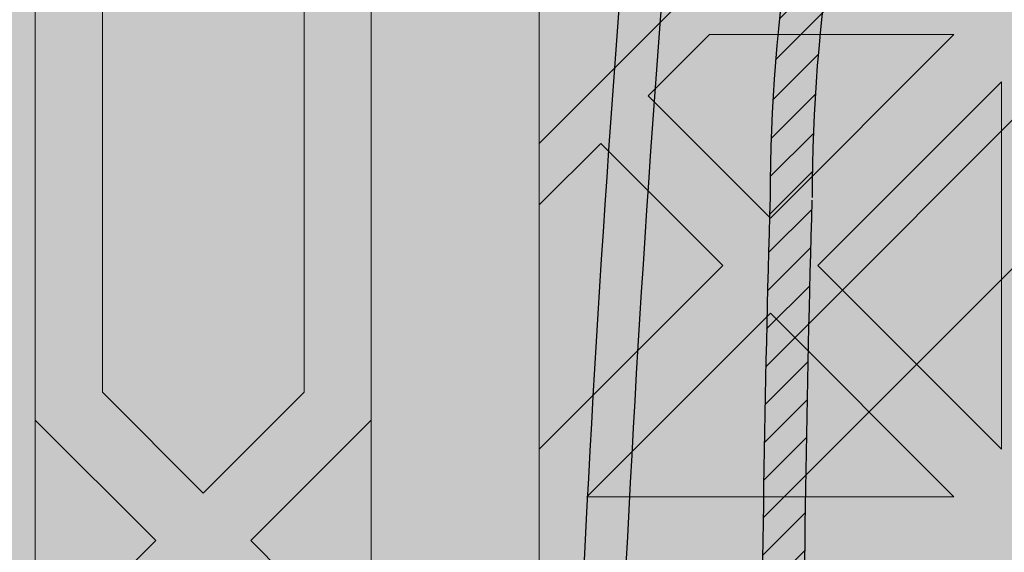
# Model space of a CAD drawing. Units: inches. Extents: x 844 to 2234, y 346 to 1084.
# Tile 16 of 93: x 1116.421 to 1120.159, y 699.229 to 701.25. Entities that reach past the tile are written whole.
import ezdxf

# ---------------------------------------------------------------- set-up
doc = ezdxf.new("R2010")
doc.units = ezdxf.units.IN
doc.header["$MEASUREMENT"] = 0
for name, color, linetype, lineweight in [('A-ANNO-DIMS', 2, 'Continuous', 18), ('furniture', 8, 'Continuous', 18), ('RA-AP-01$0$INT', 35, 'Continuous', 5)]:
    doc.layers.add(name, color=color, linetype=linetype, lineweight=lineweight)
doc.layers.add('RA-AP-01$0$FURN', color=3, linetype='Continuous')
doc.layers.add('RA-AP-01$0$WOOD', color=64, linetype='Continuous')
doc.styles.get("Standard").update_dxf_attribs({"font": 'arial.ttf'})
doc.dimstyles.get("Standard").update_dxf_attribs({"dimtxt": 6, "dimasz": 3, "dimexe": 0.18, "dimexo": 0.0625, "dimgap": 0.09, "dimtad": 0, "dimtih": 1, "dimtoh": 1, "dimdec": 1, "dimzin": 0, "dimdsep": 46, "dimlunit": 3, "dimtxsty": 'Standard', "dimblk": 'ARCHTICK', "dimcen": 0.09, "dimadec": 0, "dimazin": 0, "dimtfac": 1, "dimtdec": 1, "dimtofl": 0, "dimtmove": 0, "dimatfit": 3, "dimfxl": 1, "dimtolj": 1, "dimtzin": 0, "dimarcsym": 0})

# ---------------------------------------------------------------- blocks, each defined once
blk = doc.blocks.new('A$C18D01794')
at = {"layer": 'RA-AP-01$0$INT'}
h = blk.add_hatch(color=256, dxfattribs=at)
h.paths.add_polyline_path([(4.35521, -6.15671), (4.35521, -8.05671), (5.45521, -8.05671), (5.45521, -6.15671)])
h.paths.add_polyline_path([(4.40521, -8.00671), (4.40521, -6.20671), (5.40521, -6.20671), (5.40521, -8.00671)], flags=16)
h = blk.add_hatch(color=256, dxfattribs=at)
h.paths.add_polyline_path([(4.50521, -7.5855), (4.46935, -7.54964), (4.50521, -7.51378), (4.50521, -7.38196), (4.46935, -7.34611), (4.50521, -7.31025), (4.50521, -7.17843), (4.46935, -7.14257), (4.50521, -7.10671), (4.47692, -7.10671), (4.45521, -7.12843), (4.43349, -7.10671), (4.40521, -7.10671), (4.44106, -7.14257), (4.40521, -7.17843), (4.40521, -7.31025), (4.44106, -7.34611), (4.40521, -7.38196), (4.40521, -7.51378), (4.44106, -7.54964), (4.40521, -7.5855), (4.40521, -7.71732), (4.44106, -7.75318), (4.40521, -7.78903), (4.40521, -8.00671), (4.64435, -8.00671), (4.68021, -7.97085), (4.71606, -8.00671), (4.86935, -8.00671), (4.90521, -7.97085), (4.94106, -8.00671), (5.09435, -8.00671), (5.13021, -7.97085), (5.16606, -8.00671), (5.40521, -8.00671), (5.40521, -7.78903), (5.36935, -7.75318), (5.40521, -7.71732), (5.40521, -7.5855), (5.36935, -7.54964), (5.40521, -7.51378), (5.40521, -7.38196), (5.36935, -7.34611), (5.40521, -7.31025), (5.40521, -7.17843), (5.36935, -7.14257), (5.40521, -7.10671), (5.37692, -7.10671), (5.35521, -7.12843), (5.33349, -7.10671), (5.30521, -7.10671), (5.34106, -7.14257), (5.30521, -7.17843), (5.30521, -7.31025), (5.34106, -7.34611), (5.30521, -7.38196), (5.30521, -7.51378), (5.34106, -7.54964), (5.30521, -7.5855), (5.30521, -7.71732), (5.34106, -7.75318), (5.30521, -7.78903), (5.30521, -7.90671), (5.16606, -7.90671), (5.13021, -7.94257), (5.09435, -7.90671), (4.94106, -7.90671), (4.90521, -7.94257), (4.86935, -7.90671), (4.71606, -7.90671), (4.68021, -7.94257), (4.64435, -7.90671), (4.50521, -7.90671), (4.50521, -7.78903), (4.46935, -7.75318), (4.50521, -7.71732)])
h.paths.add_polyline_path([(4.48521, -7.70903), (4.45521, -7.73903), (4.42521, -7.70903), (4.42521, -7.59378), (4.45521, -7.56378), (4.48521, -7.59378)], flags=16)
h.paths.add_polyline_path([(4.45521, -7.76732), (4.48521, -7.79732), (4.48521, -7.91257), (4.45521, -7.94257), (4.42521, -7.91257), (4.42521, -7.79732)], flags=16)
h.paths.add_polyline_path([(4.45521, -7.5355), (4.42521, -7.5055), (4.42521, -7.39025), (4.45521, -7.36025), (4.48521, -7.39025), (4.48521, -7.5055)], flags=16)
h.paths.add_polyline_path([(4.49935, -7.92671), (4.63606, -7.92671), (4.66606, -7.95671), (4.63606, -7.98671), (4.49935, -7.98671), (4.46935, -7.95671)], flags=16)
h.paths.add_polyline_path([(4.42521, -7.94085), (4.47106, -7.98671), (4.42521, -7.98671)], flags=16)
h.paths.add_polyline_path([(4.45521, -7.33196), (4.42521, -7.30196), (4.42521, -7.18671), (4.45521, -7.15671), (4.48521, -7.18671), (4.48521, -7.30196)], flags=16)
h.paths.add_polyline_path([(4.72435, -7.92671), (4.86106, -7.92671), (4.89106, -7.95671), (4.86106, -7.98671), (4.72435, -7.98671), (4.69435, -7.95671)], flags=16)
h.paths.add_polyline_path([(4.91935, -7.95671), (4.94935, -7.92671), (5.08606, -7.92671), (5.11606, -7.95671), (5.08606, -7.98671), (4.94935, -7.98671)], flags=16)
h.paths.add_polyline_path([(5.14435, -7.95671), (5.17435, -7.92671), (5.31106, -7.92671), (5.34106, -7.95671), (5.31106, -7.98671), (5.17435, -7.98671)], flags=16)
h.paths.add_polyline_path([(5.32521, -7.59378), (5.35521, -7.56378), (5.38521, -7.59378), (5.38521, -7.70903), (5.35521, -7.73903), (5.32521, -7.70903)], flags=16)
h.paths.add_polyline_path([(5.32521, -7.79732), (5.35521, -7.76732), (5.38521, -7.79732), (5.38521, -7.91257), (5.35521, -7.94257), (5.32521, -7.91257)], flags=16)
h.paths.add_polyline_path([(5.32521, -7.5055), (5.32521, -7.39025), (5.35521, -7.36025), (5.38521, -7.39025), (5.38521, -7.5055), (5.35521, -7.5355)], flags=16)
h.paths.add_polyline_path([(5.32521, -7.30196), (5.32521, -7.18671), (5.35521, -7.15671), (5.38521, -7.18671), (5.38521, -7.30196), (5.35521, -7.33196)], flags=16)
h.paths.add_polyline_path([(5.33935, -7.98671), (5.38521, -7.94085), (5.38521, -7.98671)], flags=16)
h = blk.add_hatch(color=256, dxfattribs=at)
h.paths.add_polyline_path([(4.46935, -7.14257), (4.50521, -7.17843), (4.50521, -7.10671)])
h.paths.add_polyline_path([(4.45521, -7.12843), (4.47692, -7.10671), (4.43349, -7.10671)])
h.paths.add_polyline_path([(4.40521, -7.17843), (4.44106, -7.14257), (4.40521, -7.10671)])
h.paths.add_polyline_path([(4.42521, -7.30196), (4.45521, -7.33196), (4.48521, -7.30196), (4.48521, -7.18671), (4.45521, -7.15671), (4.42521, -7.18671)])
h.paths.add_polyline_path([(4.50521, -7.38196), (4.50521, -7.31025), (4.46935, -7.34611)])
h.paths.add_polyline_path([(4.42521, -7.5055), (4.45521, -7.5355), (4.48521, -7.5055), (4.48521, -7.39025), (4.45521, -7.36025), (4.42521, -7.39025)])
h.paths.add_polyline_path([(4.42521, -7.70903), (4.45521, -7.73903), (4.48521, -7.70903), (4.48521, -7.59378), (4.45521, -7.56378), (4.42521, -7.59378)])
h.paths.add_polyline_path([(4.46935, -7.54964), (4.50521, -7.5855), (4.50521, -7.51378)])
h.paths.add_polyline_path([(4.40521, -7.5855), (4.44106, -7.54964), (4.40521, -7.51378)])
h.paths.add_polyline_path([(4.40521, -7.78903), (4.44106, -7.75318), (4.40521, -7.71732)])
h.paths.add_polyline_path([(4.46935, -7.75318), (4.50521, -7.78903), (4.50521, -7.71732)])
h.paths.add_polyline_path([(4.42521, -7.91257), (4.45521, -7.94257), (4.48521, -7.91257), (4.48521, -7.79732), (4.45521, -7.76732), (4.42521, -7.79732)])
h.paths.add_polyline_path([(4.42521, -7.98671), (4.47106, -7.98671), (4.42521, -7.94085)])
h.paths.add_polyline_path([(4.49935, -7.98671), (4.63606, -7.98671), (4.66606, -7.95671), (4.63606, -7.92671), (4.49935, -7.92671), (4.46935, -7.95671)])
h.paths.add_polyline_path([(4.68021, -7.94257), (4.71606, -7.90671), (4.64435, -7.90671)])
h.paths.add_polyline_path([(4.64435, -8.00671), (4.71606, -8.00671), (4.68021, -7.97085)])
h.paths.add_polyline_path([(4.72435, -7.98671), (4.86106, -7.98671), (4.89106, -7.95671), (4.86106, -7.92671), (4.72435, -7.92671), (4.69435, -7.95671)])
h.paths.add_polyline_path([(4.90521, -7.94257), (4.94106, -7.90671), (4.86935, -7.90671)])
h.paths.add_polyline_path([(4.86935, -8.00671), (4.94106, -8.00671), (4.90521, -7.97085)])
h.paths.add_polyline_path([(4.94935, -7.98671), (5.08606, -7.98671), (5.11606, -7.95671), (5.08606, -7.92671), (4.94935, -7.92671), (4.91935, -7.95671)])
h.paths.add_polyline_path([(5.13021, -7.94257), (5.16606, -7.90671), (5.09435, -7.90671)])
h.paths.add_polyline_path([(5.09435, -8.00671), (5.16606, -8.00671), (5.13021, -7.97085)])
h.paths.add_polyline_path([(5.17435, -7.98671), (5.31106, -7.98671), (5.34106, -7.95671), (5.31106, -7.92671), (5.17435, -7.92671), (5.14435, -7.95671)])
h.paths.add_polyline_path([(5.32521, -7.91257), (5.35521, -7.94257), (5.38521, -7.91257), (5.38521, -7.79732), (5.35521, -7.76732), (5.32521, -7.79732)])
h.paths.add_polyline_path([(5.33935, -7.98671), (5.38521, -7.98671), (5.38521, -7.94085)])
h.paths.add_polyline_path([(5.32521, -7.70903), (5.35521, -7.73903), (5.38521, -7.70903), (5.38521, -7.59378), (5.35521, -7.56378), (5.32521, -7.59378)])
h.paths.add_polyline_path([(5.30521, -7.78903), (5.34106, -7.75318), (5.30521, -7.71732)])
h.paths.add_polyline_path([(5.36935, -7.75318), (5.40521, -7.78903), (5.40521, -7.71732)])
h.paths.add_polyline_path([(5.40521, -7.5855), (5.40521, -7.51378), (5.36935, -7.54964)])
h.paths.add_polyline_path([(5.30521, -7.5855), (5.34106, -7.54964), (5.30521, -7.51378)])
h.paths.add_polyline_path([(5.32521, -7.5055), (5.35521, -7.5355), (5.38521, -7.5055), (5.38521, -7.39025), (5.35521, -7.36025), (5.32521, -7.39025)])
h.paths.add_polyline_path([(5.30521, -7.38196), (5.34106, -7.34611), (5.30521, -7.31025)])
h.paths.add_polyline_path([(5.32521, -7.30196), (5.35521, -7.33196), (5.38521, -7.30196), (5.38521, -7.18671), (5.35521, -7.15671), (5.32521, -7.18671)])
h.paths.add_polyline_path([(5.40458, -7.38134, -0.001218), (5.40521, -7.38111), (5.40521, -7.31025), (5.36935, -7.34611)])
h.paths.add_polyline_path([(5.36935, -7.14257), (5.40521, -7.17843), (5.40521, -7.10671)])
h.paths.add_polyline_path([(5.35521, -7.12843), (5.37692, -7.10671), (5.33349, -7.10671)])
h.paths.add_polyline_path([(5.30521, -7.17843), (5.34106, -7.14257), (5.30521, -7.10671)])
for points in [[(4.50521, -7.90671), (5.30521, -7.90671), (5.30521, -7.10671), (5.25521, -7.10671), (5.25521, -7.85671), (4.55521, -7.85671), (4.55521, -7.10671), (4.50521, -7.10671)], [(4.40521, -7.38196), (4.44106, -7.34611), (4.40521, -7.31025)]]:
    blk.add_hatch(color=256, dxfattribs=at).paths.add_polyline_path(points)
h = blk.add_hatch(color=256, dxfattribs=at)
h.paths.add_polyline_path([(4.58592, -7.85671), (4.6142, -7.85671), (4.66885, -7.80207), (4.72349, -7.85671), (4.77177, -7.85671), (4.82642, -7.80207), (4.86278, -7.83843), (4.8445, -7.85671), (4.86278, -7.85671), (4.90521, -7.81429), (4.94763, -7.85671), (4.96592, -7.85671), (4.94763, -7.83843), (4.98399, -7.80207), (5.03864, -7.85671), (5.08692, -7.85671), (5.14157, -7.80207), (5.19621, -7.85671), (5.2245, -7.85671), (4.90521, -7.53742)])
h.paths.add_polyline_path([(4.89521, -7.57571), (4.89521, -7.685), (4.84056, -7.63035)], flags=16)
h.paths.add_polyline_path([(4.91521, -7.57571), (4.96985, -7.63035), (4.91521, -7.685)], flags=16)
h.paths.add_polyline_path([(4.82642, -7.64449), (4.88106, -7.69914), (4.77177, -7.69914)], flags=16)
h.paths.add_polyline_path([(4.98399, -7.64449), (5.03864, -7.69914), (4.92935, -7.69914)], flags=16)
h.paths.add_polyline_path([(4.88106, -7.71914), (4.82642, -7.77378), (4.77177, -7.71914)], flags=16)
h.paths.add_polyline_path([(4.92935, -7.71914), (5.03864, -7.71914), (4.98399, -7.77378)], flags=16)
h.paths.add_polyline_path([(4.89521, -7.73328), (4.89521, -7.806), (4.87692, -7.82429), (4.84056, -7.78793)], flags=16)
h.paths.add_polyline_path([(4.91521, -7.73328), (4.96985, -7.78793), (4.93349, -7.82429), (4.91521, -7.806)], flags=16)
h.paths.add_polyline_path([(4.75763, -7.73328), (4.81228, -7.78793), (4.75763, -7.84257)], flags=16)
h.paths.add_polyline_path([(4.73763, -7.73328), (4.73763, -7.84257), (4.68299, -7.78793)], flags=16)
h.paths.add_polyline_path([(5.05278, -7.73328), (5.05278, -7.84257), (4.99814, -7.78793)], flags=16)
h.paths.add_polyline_path([(5.07278, -7.73328), (5.12742, -7.78793), (5.07278, -7.84257)], flags=16)
h.paths.add_polyline_path([(4.93592, -7.50671), (5.25521, -7.826), (5.25521, -7.79772), (5.20056, -7.74307), (5.25521, -7.68843), (5.25521, -7.64014), (5.20056, -7.5855), (5.23692, -7.54914), (5.25521, -7.56742), (5.25521, -7.54914), (5.21278, -7.50671), (5.25521, -7.46429), (5.25521, -7.446), (5.23692, -7.46429), (5.20056, -7.42793), (5.25521, -7.37328), (5.25521, -7.325), (5.20056, -7.27035), (5.25521, -7.21571), (5.25521, -7.18742)])
h.paths.add_polyline_path([(5.04299, -7.42793), (5.09763, -7.37328), (5.09763, -7.48257)], flags=16)
h.paths.add_polyline_path([(5.02885, -7.44207), (5.08349, -7.49671), (4.9742, -7.49671)], flags=16)
h.paths.add_polyline_path([(5.11763, -7.37328), (5.17228, -7.42793), (5.11763, -7.48257)], flags=16)
h.paths.add_polyline_path([(5.08349, -7.51671), (5.02885, -7.57136), (4.9742, -7.51671)], flags=16)
h.paths.add_polyline_path([(5.13177, -7.35914), (5.18642, -7.41378), (5.24106, -7.35914)], flags=17)
h.paths.add_polyline_path([(5.13177, -7.49671), (5.18642, -7.44207), (5.22278, -7.47843), (5.2045, -7.49671)], flags=16)
h.paths.add_polyline_path([(5.09763, -7.53085), (5.09763, -7.64014), (5.04299, -7.5855)], flags=16)
h.paths.add_polyline_path([(5.13177, -7.33914), (5.24106, -7.33914), (5.18642, -7.28449)], flags=17)
h.paths.add_polyline_path([(5.13177, -7.51671), (5.2045, -7.51671), (5.22278, -7.535), (5.18642, -7.57136)], flags=16)
h.paths.add_polyline_path([(5.11763, -7.53085), (5.17228, -7.5855), (5.11763, -7.64014)], flags=16)
h.paths.add_polyline_path([(5.18642, -7.59964), (5.24106, -7.65429), (5.13177, -7.65429)], flags=16)
h.paths.add_polyline_path([(5.13177, -7.67429), (5.24106, -7.67429), (5.18642, -7.72893)], flags=16)
h.paths.add_polyline_path([(5.25521, -7.126), (5.25521, -7.10671), (4.55521, -7.10671), (4.55521, -7.126), (4.90521, -7.476)])
h.paths.add_polyline_path([(4.98399, -7.36893), (4.92935, -7.31429), (5.03864, -7.31429)], flags=16)
h.paths.add_polyline_path([(4.96985, -7.38307), (4.91521, -7.43772), (4.91521, -7.32843)], flags=16)
h.paths.add_polyline_path([(4.92935, -7.29429), (4.98399, -7.23964), (5.03864, -7.29429)], flags=16)
h.paths.add_polyline_path([(5.05278, -7.28014), (4.99814, -7.2255), (5.05278, -7.17085)], flags=16)
h.paths.add_polyline_path([(5.07278, -7.28014), (5.07278, -7.17085), (5.12742, -7.2255)], flags=16)
h.paths.add_polyline_path([(4.89521, -7.43772), (4.84056, -7.38307), (4.89521, -7.32843)], flags=16)
h.paths.add_polyline_path([(4.91521, -7.28014), (4.91521, -7.20742), (4.93349, -7.18914), (4.96985, -7.2255)], flags=16)
h.paths.add_polyline_path([(4.88106, -7.31429), (4.82642, -7.36893), (4.77177, -7.31429)], flags=16)
h.paths.add_polyline_path([(4.89521, -7.28014), (4.84056, -7.2255), (4.87692, -7.18914), (4.89521, -7.20742)], flags=16)
h.paths.add_polyline_path([(4.98399, -7.21136), (4.94763, -7.175), (4.96592, -7.15671), (5.03864, -7.15671)], flags=16)
h.paths.add_polyline_path([(4.88106, -7.29429), (4.77177, -7.29429), (4.82642, -7.23964)], flags=16)
h.paths.add_polyline_path([(4.90521, -7.19914), (4.86278, -7.15671), (4.94763, -7.15671)], flags=16)
h.paths.add_polyline_path([(5.14157, -7.21136), (5.08692, -7.15671), (5.19621, -7.15671)], flags=16)
h.paths.add_polyline_path([(4.82642, -7.21136), (4.77177, -7.15671), (4.8445, -7.15671), (4.86278, -7.175)], flags=16)
h.paths.add_polyline_path([(4.81228, -7.2255), (4.75763, -7.28014), (4.75763, -7.17085)], flags=16)
h.paths.add_polyline_path([(4.73763, -7.28014), (4.68299, -7.2255), (4.73763, -7.17085)], flags=16)
h.paths.add_polyline_path([(4.72349, -7.15671), (4.66885, -7.21136), (4.6142, -7.15671)], flags=16)
h.paths.add_polyline_path([(4.59763, -7.50671), (4.55521, -7.54914), (4.55521, -7.56742), (4.57349, -7.54914), (4.60985, -7.5855), (4.55521, -7.64014), (4.55521, -7.68843), (4.60985, -7.74307), (4.55521, -7.79772), (4.55521, -7.826), (4.8745, -7.50671), (4.55521, -7.18742), (4.55521, -7.21571), (4.60985, -7.27035), (4.55521, -7.325), (4.55521, -7.37328), (4.60985, -7.42793), (4.57349, -7.46429), (4.55521, -7.446), (4.55521, -7.46429)])
h.paths.add_polyline_path([(4.71278, -7.48257), (4.71278, -7.37328), (4.76742, -7.42793)], flags=16)
h.paths.add_polyline_path([(4.72692, -7.49671), (4.78157, -7.44207), (4.83621, -7.49671)], flags=16)
h.paths.add_polyline_path([(4.69278, -7.48257), (4.63814, -7.42793), (4.69278, -7.37328)], flags=16)
h.paths.add_polyline_path([(4.72692, -7.51671), (4.83621, -7.51671), (4.78157, -7.57136)], flags=16)
h.paths.add_polyline_path([(4.67864, -7.49671), (4.60592, -7.49671), (4.58763, -7.47843), (4.62399, -7.44207)], flags=16)
h.paths.add_polyline_path([(4.71278, -7.53085), (4.76742, -7.5855), (4.71278, -7.64014)], flags=16)
h.paths.add_polyline_path([(4.67864, -7.51671), (4.62399, -7.57136), (4.58763, -7.535), (4.60592, -7.51671)], flags=16)
h.paths.add_polyline_path([(4.69278, -7.53085), (4.69278, -7.64014), (4.63814, -7.5855)], flags=16)
h.paths.add_polyline_path([(4.62399, -7.41378), (4.67864, -7.35914), (4.56935, -7.35914)], flags=17)
h.paths.add_polyline_path([(4.62399, -7.59964), (4.67864, -7.65429), (4.56935, -7.65429)], flags=16)
h.paths.add_polyline_path([(4.67864, -7.33914), (4.62399, -7.28449), (4.56935, -7.33914)], flags=17)
h.paths.add_polyline_path([(4.67864, -7.67429), (4.62399, -7.72893), (4.56935, -7.67429)], flags=16)
h = blk.add_hatch(color=256, dxfattribs=at)
h.paths.add_polyline_path([(4.78157, -7.44207), (4.83621, -7.49671), (4.72692, -7.49671)])
h.paths.add_polyline_path([(4.83621, -7.51671), (4.78157, -7.57136), (4.72692, -7.51671)])
h.paths.add_polyline_path([(4.76742, -7.5855), (4.71278, -7.64014), (4.71278, -7.53085)])
h.paths.add_polyline_path([(4.69278, -7.53085), (4.69278, -7.64014), (4.63814, -7.5855)])
h.paths.add_polyline_path([(4.67864, -7.51671), (4.62399, -7.57136), (4.58763, -7.535), (4.60592, -7.51671)])
h.paths.add_polyline_path([(4.57349, -7.54914), (4.60985, -7.5855), (4.55521, -7.64014), (4.55521, -7.56742)])
h.paths.add_polyline_path([(4.62399, -7.59964), (4.67864, -7.65429), (4.56935, -7.65429)])
h.paths.add_polyline_path([(4.67864, -7.67429), (4.62399, -7.72893), (4.56935, -7.67429)])
h.paths.add_polyline_path([(4.60985, -7.74307), (4.55521, -7.79772), (4.55521, -7.68843)])
h.paths.add_polyline_path([(4.59763, -7.50671), (4.55521, -7.54914), (4.55521, -7.46429)])
h.paths.add_polyline_path([(4.67864, -7.49671), (4.60592, -7.49671), (4.58763, -7.47843), (4.62399, -7.44207)])
h.paths.add_polyline_path([(4.69278, -7.37328), (4.69278, -7.48257), (4.63814, -7.42793)])
h.paths.add_polyline_path([(4.76742, -7.42793), (4.71278, -7.48257), (4.71278, -7.37328)])
h.paths.add_polyline_path([(4.67864, -7.35914), (4.62399, -7.41378), (4.56935, -7.35914)])
h.paths.add_polyline_path([(4.60985, -7.42793), (4.57349, -7.46429), (4.55521, -7.446), (4.55521, -7.37328)])
h.paths.add_polyline_path([(4.62399, -7.28449), (4.67864, -7.33914), (4.56935, -7.33914)])
h.paths.add_polyline_path([(4.60985, -7.27035), (4.55521, -7.325), (4.55521, -7.21571)])
for p, q in [((4.55521, -7.10671), (4.55521, -7.85671)), ((4.40521, -7.31025), (4.44106, -7.34611)), ((4.50521, -7.31025), (4.46935, -7.34611)), ((4.40521, -7.38196), (4.44106, -7.34611)), ((4.50521, -7.38196), (4.46935, -7.34611)), ((4.42521, -7.39025), (4.45521, -7.36025)), ((4.48521, -7.39025), (4.45521, -7.36025)), ((4.67864, -7.35914), (4.56935, -7.35914)), ((4.56935, -7.35914), (4.62399, -7.41378)), ((4.67864, -7.35914), (4.62399, -7.41378)), ((4.55521, -7.446), (4.55521, -7.37328)), ((4.55521, -7.37328), (4.60985, -7.42793)), ((4.69278, -7.37328), (4.63814, -7.42793)), ((4.69278, -7.37328), (4.69278, -7.48257)), ((4.42521, -7.39025), (4.42521, -7.5055)), ((4.48521, -7.39025), (4.48521, -7.5055)), ((4.60985, -7.42793), (4.57349, -7.46429)), ((4.69278, -7.48257), (4.63814, -7.42793)), ((4.62399, -7.44207), (4.58763, -7.47843)), ((4.67864, -7.49671), (4.62399, -7.44207)), ((4.55521, -7.446), (4.57349, -7.46429)), ((4.57349, -7.46429), (4.55521, -7.446)), ((4.59763, -7.50671), (4.55521, -7.46429)), ((4.55521, -7.46429), (4.55521, -7.54914)), ((4.60592, -7.49671), (4.58763, -7.47843)), ((4.60592, -7.49671), (4.67864, -7.49671))]:
    blk.add_line(p, q, dxfattribs=at)
for points in [[(5.40521, -8.00671), (4.40521, -8.00671), (4.40521, -7.10671)], [(5.30521, -7.10671), (5.30521, -7.90671), (4.50521, -7.90671), (4.50521, -7.10671)]]:
    blk.add_lwpolyline(points, dxfattribs=at)
blk = doc.blocks.new('A$C32926AE1')
at = {"layer": 'RA-AP-01$0$WOOD'}
h = blk.add_hatch(color=256, dxfattribs=at)
h.dxf.hatch_style = 1
h.paths.add_polyline_path([(5.15743, 4.57348, -0.100949), (5.1554, 4.59337, -0.184266), (5.17225, 4.6388, 0.205661), (5.17956, 4.66132, 0.361434), (5.13435, 4.70652, 0.205661), (5.11183, 4.69921, -0.184266), (5.0664, 4.68237, -0.105531), (5.04566, 4.68467, 0.156764), (4.76389, 4.68467, -0.105531), (4.74314, 4.68237, -0.184266), (4.69771, 4.69921, 0.205661), (4.67519, 4.70652, 0.361434), (4.62998, 4.66132, 0.205661), (4.63729, 4.6388, -0.184266), (4.65414, 4.59337, -0.100949), (4.65211, 4.57348, 0.02141), (4.62975, 4.15671, 0.02141), (4.65211, 3.73994, -0.100949), (4.65414, 3.72006, -0.184266), (4.63729, 3.67463, 0.205661), (4.62998, 3.65211, 0.361434), (4.67519, 3.6069, 0.205661), (4.69771, 3.61421, -0.184266), (4.74314, 3.63106, -0.105531), (4.76389, 3.62875, 0.156764), (5.04566, 3.62875, -0.105531), (5.0664, 3.63106, -0.184266), (5.11183, 3.61421, 0.205661), (5.13435, 3.6069, 0.361434), (5.17956, 3.65211, 0.205661), (5.17225, 3.67463, -0.184266), (5.1554, 3.72006, -0.100949), (5.15743, 3.73994, 0.02141), (5.17979, 4.15671, 0.02141)])
h.paths.add_polyline_path([(4.63975, 4.15671, 0.021354), (4.66197, 3.74189, -0.094076), (4.66414, 3.71961, -0.182482), (4.64481, 3.66804, 0.205661), (4.63994, 3.65302, 0.361434), (4.67611, 3.61686, 0.205661), (4.69112, 3.62173, -0.182482), (4.7427, 3.64106, -0.102989), (4.76699, 3.63826, 0.156709), (5.04255, 3.63826, -0.102989), (5.06685, 3.64106, -0.182482), (5.11842, 3.62173, 0.205661), (5.13344, 3.61686, 0.361434), (5.1696, 3.65302, 0.205661), (5.16473, 3.66804, -0.182482), (5.1454, 3.71961, -0.094076), (5.14757, 3.74189, 0.021354), (5.16979, 4.15671, 0.021354), (5.14757, 4.57154, -0.094076), (5.1454, 4.59381, -0.182482), (5.16473, 4.64539, 0.205661), (5.1696, 4.6604, 0.361434), (5.13344, 4.69657, 0.205661), (5.11842, 4.69169, -0.182482), (5.06685, 4.67236, -0.102989), (5.04255, 4.67517, 0.156709), (4.76699, 4.67517, -0.102989), (4.7427, 4.67236, -0.182482), (4.69112, 4.69169, 0.205661), (4.67611, 4.69657, 0.361434), (4.63994, 4.6604, 0.205661), (4.64481, 4.64539, -0.182482), (4.66414, 4.59381, -0.094076), (4.66197, 4.57154, 0.021354)], flags=16)
h.paths.add_polyline_path([(5.12979, 4.43217, -0.014166), (5.13015, 4.15693, -0.014166), (5.12979, 3.88169, -0.078525), (5.1098, 3.75514, 0.094597), (5.10541, 3.7179, 0.104317), (5.11607, 3.67039, 0.104317), (5.06856, 3.68105, 0.094597), (5.03132, 3.67666, -0.158024), (4.77823, 3.67666, 0.094597), (4.74098, 3.68105, 0.104317), (4.69347, 3.67039, 0.104317), (4.70413, 3.7179, 0.094597), (4.69975, 3.75514, -0.078525), (4.67975, 3.88169, -0.014166), (4.67939, 4.15693, -0.014166), (4.67975, 4.43217, -0.078525), (4.69975, 4.55871, 0.094597), (4.70413, 4.59596, 0.104317), (4.69347, 4.64347, 0.104317), (4.74098, 4.6328, 0.094597), (4.77823, 4.63719, -0.158024), (5.03132, 4.63719, 0.094597), (5.06856, 4.6328, 0.104317), (5.11607, 4.64347, 0.104317), (5.10541, 4.59596, 0.094597), (5.1098, 4.55871, -0.078525)], flags=0)
h.paths.add_polyline_path([(5.11979, 4.43226, -0.0142), (5.12016, 4.15693, -0.0142), (5.11979, 3.8816, -0.078489), (5.10027, 3.75819, 0.094014), (5.09541, 3.71748, 0.060627), (5.09962, 3.68684, 0.060627), (5.06898, 3.69105, 0.094014), (5.02827, 3.68619, -0.158071), (4.78127, 3.68619, 0.094014), (4.74056, 3.69105, 0.060627), (4.70993, 3.68684, 0.060627), (4.71413, 3.71748, 0.094014), (4.70927, 3.75819, -0.078489), (4.68975, 3.8816, -0.0142), (4.68939, 4.15693, -0.0142), (4.68975, 4.43226, -0.078489), (4.70927, 4.55566, 0.094014), (4.71413, 4.59638, 0.060627), (4.70993, 4.62701, 0.060627), (4.74056, 4.62281, 0.094014), (4.78127, 4.62767, -0.158071), (5.02827, 4.62767, 0.094014), (5.06898, 4.62281, 0.060627), (5.09962, 4.62701, 0.060627), (5.09541, 4.59638, 0.094014), (5.10027, 4.55566, -0.078489)], flags=0)
h.paths.add_polyline_path([(5.06979, 4.43022, -0.014242), (5.07017, 4.15693, -0.014242), (5.06979, 3.88364, -0.080061), (5.05266, 3.77346, 0.052642), (5.04591, 3.74055, 0.052642), (5.013, 3.7338, -0.158303), (4.79655, 3.7338, 0.052642), (4.76363, 3.74055, 0.052642), (4.75688, 3.77346, -0.080061), (4.73975, 3.88364, -0.014242), (4.73937, 4.15693, -0.014242), (4.73975, 4.43022, -0.080061), (4.75688, 4.54039, 0.052642), (4.76363, 4.5733, 0.052642), (4.79655, 4.58006, -0.158303), (5.013, 4.58006, 0.052642), (5.04591, 4.5733, 0.052642), (5.05266, 4.54039, -0.080061)], flags=0)
h.paths.add_polyline_path([(5.04979, 4.43038, -0.01431), (5.05018, 4.15693, -0.01431), (5.04979, 3.88347, -0.080069), (5.03362, 3.77958, 0.030626), (5.02824, 3.75822, 0.030626), (5.00688, 3.75284, -0.158398), (4.80266, 3.75284, 0.030626), (4.7813, 3.75822, 0.030626), (4.77592, 3.77958, -0.080069), (4.75975, 3.88347, -0.01431), (4.75936, 4.15693, -0.01431), (4.75975, 4.43038, -0.080069), (4.77592, 4.53427, 0.030626), (4.7813, 4.55564, 0.030626), (4.80266, 4.56102, -0.158398), (5.00688, 4.56102, 0.030626), (5.02824, 4.55564, 0.030626), (5.03362, 4.53427, -0.080069)], flags=0)
h.paths.add_polyline_path([(4.99977, 4.42817, -0.014344), (5.0002, 4.15693, -0.014344), (4.99977, 3.88568, -0.078464), (4.98736, 3.7991, -0.150605), (4.82219, 3.7991, -0.078464), (4.80978, 3.88568, -0.014344), (4.80934, 4.15693, -0.014344), (4.80978, 4.42817, -0.078464), (4.82219, 4.51475, -0.150605), (4.98736, 4.51475, -0.078464)], flags=0)
h.paths.add_polyline_path([(4.97976, 4.42764, -0.014377), (4.98021, 4.15693, -0.014377), (4.97976, 3.88621, -0.068924), (4.97118, 3.81528, -0.129665), (4.83836, 3.81528, -0.068924), (4.82979, 3.88621, -0.014377), (4.82934, 4.15693, -0.014377), (4.82979, 4.42764, -0.068924), (4.83836, 4.49858, -0.129665), (4.97118, 4.49858, -0.068924)], flags=0)
h = blk.add_hatch(color=256, dxfattribs=at)
h.dxf.hatch_style = 1
h.paths.add_polyline_path([(5.1454, 4.59381, -0.182482), (5.16473, 4.64539, 0.205661), (5.1696, 4.6604, 0.361434), (5.13344, 4.69657, 0.205661), (5.11842, 4.69169, -0.182482), (5.06685, 4.67236, -0.102989), (5.04255, 4.67517, 0.156709), (4.76699, 4.67517, -0.102989), (4.7427, 4.67236, -0.182482), (4.69112, 4.69169, 0.205661), (4.67611, 4.69657, 0.361434), (4.63994, 4.6604, 0.205661), (4.64481, 4.64539, -0.182482), (4.66414, 4.59381, -0.094076), (4.66197, 4.57154, 0.021354), (4.63975, 4.15671, 0.021354), (4.66197, 3.74189, -0.094076), (4.66414, 3.71961, -0.182482), (4.64481, 3.66804, 0.205661), (4.63994, 3.65302, 0.361434), (4.67611, 3.61686, 0.205661), (4.69112, 3.62173, -0.182482), (4.7427, 3.64106, -0.102989), (4.76699, 3.63826, 0.156709), (5.04255, 3.63826, -0.102989), (5.06685, 3.64106, -0.182482), (5.11842, 3.62173, 0.205661), (5.13344, 3.61686, 0.361434), (5.1696, 3.65302, 0.205661), (5.16473, 3.66804, -0.182482), (5.1454, 3.71961, -0.094076), (5.14757, 3.74189, 0.021354), (5.16979, 4.15671, 0.021354), (5.14757, 4.57154, -0.094076)])
h.paths.add_polyline_path([(5.1098, 4.55871, -0.078525), (5.12979, 4.43217, -0.014166), (5.13015, 4.15693, -0.014166), (5.12979, 3.88169, -0.078525), (5.1098, 3.75514, 0.094597), (5.10541, 3.7179, 0.104317), (5.11607, 3.67039, 0.104317), (5.06856, 3.68105, 0.094597), (5.03132, 3.67666, -0.158024), (4.77823, 3.67666, 0.094597), (4.74098, 3.68105, 0.104317), (4.69347, 3.67039, 0.104317), (4.70413, 3.7179, 0.094597), (4.69975, 3.75514, -0.078525), (4.67975, 3.88169, -0.014166), (4.67939, 4.15693, -0.014166), (4.67975, 4.43217, -0.078525), (4.69975, 4.55871, 0.094597), (4.70413, 4.59596, 0.104317), (4.69347, 4.64347, 0.104317), (4.74098, 4.6328, 0.094597), (4.77823, 4.63719, -0.158024), (5.03132, 4.63719, 0.094597), (5.06856, 4.6328, 0.104317), (5.11607, 4.64347, 0.104317), (5.10541, 4.59596, 0.094597)], flags=16)
h.paths.add_polyline_path([(5.10027, 4.55566, -0.078489), (5.11979, 4.43226, -0.0142), (5.12016, 4.15693, -0.0142), (5.11979, 3.8816, -0.078489), (5.10027, 3.75819, 0.094014), (5.09541, 3.71748, 0.060627), (5.09962, 3.68684, 0.060627), (5.06898, 3.69105, 0.094014), (5.02827, 3.68619, -0.158071), (4.78127, 3.68619, 0.094014), (4.74056, 3.69105, 0.060627), (4.70993, 3.68684, 0.060627), (4.71413, 3.71748, 0.094014), (4.70927, 3.75819, -0.078489), (4.68975, 3.8816, -0.0142), (4.68939, 4.15693, -0.0142), (4.68975, 4.43226, -0.078489), (4.70927, 4.55566, 0.094014), (4.71413, 4.59638, 0.060627), (4.70993, 4.62701, 0.060627), (4.74056, 4.62281, 0.094014), (4.78127, 4.62767, -0.158071), (5.02827, 4.62767, 0.094014), (5.06898, 4.62281, 0.060627), (5.09962, 4.62701, 0.060627), (5.09541, 4.59638, 0.094014)], flags=0)
h.paths.add_polyline_path([(5.04591, 4.5733, 0.052642), (5.05266, 4.54039, -0.080061), (5.06979, 4.43022, -0.014242), (5.07017, 4.15693, -0.014242), (5.06979, 3.88364, -0.080061), (5.05266, 3.77346, 0.052642), (5.04591, 3.74055, 0.052642), (5.013, 3.7338, -0.158303), (4.79655, 3.7338, 0.052642), (4.76363, 3.74055, 0.052642), (4.75688, 3.77346, -0.080061), (4.73975, 3.88364, -0.014242), (4.73937, 4.15693, -0.014242), (4.73975, 4.43022, -0.080061), (4.75688, 4.54039, 0.052642), (4.76363, 4.5733, 0.052642), (4.79655, 4.58006, -0.158303), (5.013, 4.58006, 0.052642)], flags=0)
h.paths.add_polyline_path([(5.02824, 4.55564, 0.030626), (5.03362, 4.53427, -0.080069), (5.04979, 4.43038, -0.01431), (5.05018, 4.15693, -0.01431), (5.04979, 3.88347, -0.080069), (5.03362, 3.77958, 0.030626), (5.02824, 3.75822, 0.030626), (5.00688, 3.75284, -0.158398), (4.80266, 3.75284, 0.030626), (4.7813, 3.75822, 0.030626), (4.77592, 3.77958, -0.080069), (4.75975, 3.88347, -0.01431), (4.75936, 4.15693, -0.01431), (4.75975, 4.43038, -0.080069), (4.77592, 4.53427, 0.030626), (4.7813, 4.55564, 0.030626), (4.80266, 4.56102, -0.158398), (5.00688, 4.56102, 0.030626)], flags=0)
h.paths.add_polyline_path([(4.98736, 4.51475, -0.078464), (4.99977, 4.42817, -0.014344), (5.0002, 4.15693, -0.014344), (4.99977, 3.88568, -0.078464), (4.98736, 3.7991, -0.150605), (4.82219, 3.7991, -0.078464), (4.80978, 3.88568, -0.014344), (4.80934, 4.15693, -0.014344), (4.80978, 4.42817, -0.078464), (4.82219, 4.51475, -0.150605)], flags=0)
h.paths.add_polyline_path([(4.97118, 4.49858, -0.068924), (4.97976, 4.42764, -0.014377), (4.98021, 4.15693, -0.014377), (4.97976, 3.88621, -0.068924), (4.97118, 3.81528, -0.129665), (4.83836, 3.81528, -0.068924), (4.82979, 3.88621, -0.014377), (4.82934, 4.15693, -0.014377), (4.82979, 4.42764, -0.068924), (4.83836, 4.49858, -0.129665)], flags=0)
h = blk.add_hatch(dxfattribs=at)
h.set_pattern_fill('ANSI31', color=256, scale=0.05, style=0)
h.paths.add_polyline_path([(5.13015, 4.15693, 0.014166), (5.12979, 4.43217, 0.077783), (5.11017, 4.55756, -0.097652), (5.10541, 4.59596, -0.104317), (5.11607, 4.64347), (5.09962, 4.62701, 0.060627), (5.09541, 4.59638, 0.094014), (5.10027, 4.55566, -0.078489), (5.11979, 4.43226, -0.0142), (5.12016, 4.15693, -0.0142), (5.11979, 3.8816, -0.078489), (5.10027, 3.75819, 0.094014), (5.09541, 3.71748, 0.060627), (5.09962, 3.68684), (5.11607, 3.67039, -0.104317), (5.10541, 3.7179, -0.097652), (5.11017, 3.7563, 0.077783), (5.12979, 3.88169, 0.014166)])
h.paths.add_polyline_path([(5.03016, 3.67629, -0.097652), (5.06856, 3.68105, -0.104317), (5.11607, 3.67039), (5.09962, 3.68684, 0.060627), (5.06898, 3.69105, 0.094014), (5.02827, 3.68619, -0.158071), (4.78127, 3.68619, 0.094014), (4.74056, 3.69105, 0.060627), (4.70993, 3.68684), (4.69347, 3.67039, -0.104317), (4.74098, 3.68105, -0.097652), (4.77938, 3.67629, 0.156513)])
h.paths.add_polyline_path([(4.68975, 3.8816, -0.0142), (4.68939, 4.15693, -0.0142), (4.68975, 4.43226, -0.078489), (4.70927, 4.55566, 0.094014), (4.71413, 4.59638, 0.060627), (4.70993, 4.62701), (4.69347, 4.64347, -0.104317), (4.70413, 4.59596, -0.097652), (4.69937, 4.55756, 0.077783), (4.67975, 4.43217, 0.014166), (4.67939, 4.15693, 0.014166), (4.67975, 3.88169, 0.077783), (4.69937, 3.7563, -0.097652), (4.70413, 3.7179, -0.104317), (4.69347, 3.67039), (4.70993, 3.68684, 0.060627), (4.71413, 3.71748, 0.094014), (4.70927, 3.75819, -0.078489)])
h.paths.add_polyline_path([(4.77938, 4.63756, -0.097652), (4.74098, 4.6328, -0.104317), (4.69347, 4.64347), (4.70993, 4.62701, 0.060627), (4.74056, 4.62281, 0.094014), (4.78127, 4.62767, -0.158071), (5.02827, 4.62767, 0.094014), (5.06898, 4.62281, 0.060627), (5.09962, 4.62701), (5.11607, 4.64347, -0.104317), (5.06856, 4.6328, -0.097652), (5.03016, 4.63756, 0.156513)])
h = blk.add_hatch(dxfattribs=at)
h.set_pattern_fill('ANSI32', color=256, scale=0.2, style=0)
h.paths.add_polyline_path([(5.11979, 4.43226, 0.077702), (5.10066, 4.55447, -0.09689), (5.09541, 4.59638, -0.060627), (5.09962, 4.62701, -0.060627), (5.06898, 4.62281, -0.09689), (5.02707, 4.62805, 0.156466), (4.78247, 4.62805, -0.09689), (4.74056, 4.62281, -0.060627), (4.70993, 4.62701, -0.060627), (4.71413, 4.59638, -0.09689), (4.70888, 4.55447, 0.077702), (4.68975, 4.43226, 0.0142), (4.68939, 4.15693, 0.0142), (4.68975, 3.8816, 0.077702), (4.70888, 3.75939, -0.09689), (4.71413, 3.71748, -0.060627), (4.70993, 3.68684, -0.060627), (4.74056, 3.69105, -0.09689), (4.78247, 3.6858, 0.156466), (5.02707, 3.6858, -0.09689), (5.06898, 3.69105, -0.060627), (5.09962, 3.68684, -0.060627), (5.09541, 3.71748, -0.09689), (5.10066, 3.75939, 0.077702), (5.11979, 3.8816, 0.0142), (5.12016, 4.15693, 0.0142)])
h.paths.add_polyline_path([(5.07017, 4.15693, -0.014242), (5.06979, 3.88364, -0.080061), (5.05266, 3.77346, 0.052642), (5.04591, 3.74055, 0.052642), (5.013, 3.7338, -0.158303), (4.79655, 3.7338, 0.052642), (4.76363, 3.74055, 0.052642), (4.75688, 3.77346, -0.080061), (4.73975, 3.88364, -0.014242), (4.73937, 4.15693, -0.014242), (4.73975, 4.43022, -0.080061), (4.75688, 4.54039, 0.052642), (4.76363, 4.5733, 0.052642), (4.79655, 4.58006, -0.158303), (5.013, 4.58006, 0.052642), (5.04591, 4.5733, 0.052642), (5.05266, 4.54039, -0.080061), (5.06979, 4.43022, -0.014242)], flags=16)
h.paths.add_polyline_path([(5.05018, 4.15693, -0.01431), (5.04979, 3.88347, -0.080069), (5.03362, 3.77958, 0.030626), (5.02824, 3.75822, 0.030626), (5.00688, 3.75284, -0.158398), (4.80266, 3.75284, 0.030626), (4.7813, 3.75822, 0.030626), (4.77592, 3.77958, -0.080069), (4.75975, 3.88347, -0.01431), (4.75936, 4.15693, -0.01431), (4.75975, 4.43038, -0.080069), (4.77592, 4.53427, 0.030626), (4.7813, 4.55564, 0.030626), (4.80266, 4.56102, -0.158398), (5.00688, 4.56102, 0.030626), (5.02824, 4.55564, 0.030626), (5.03362, 4.53427, -0.080069), (5.04979, 4.43038, -0.01431)], flags=0)
h.paths.add_polyline_path([(5.0002, 4.15693, -0.014344), (4.99977, 3.88568, -0.078464), (4.98736, 3.7991, -0.150605), (4.82219, 3.7991, -0.078464), (4.80978, 3.88568, -0.014344), (4.80934, 4.15693, -0.014344), (4.80978, 4.42817, -0.078464), (4.82219, 4.51475, -0.150605), (4.98736, 4.51475, -0.078464), (4.99977, 4.42817, -0.014344)], flags=0)
h.paths.add_polyline_path([(4.98021, 4.15693, -0.014377), (4.97976, 3.88621, -0.068924), (4.97118, 3.81528, -0.129665), (4.83836, 3.81528, -0.068924), (4.82979, 3.88621, -0.014377), (4.82934, 4.15693, -0.014377), (4.82979, 4.42764, -0.068924), (4.83836, 4.49858, -0.129665), (4.97118, 4.49858, -0.068924), (4.97976, 4.42764, -0.014377)], flags=0)
for centre, radius, start, end in [((9.50522, 4.10408), 4.87575, 174.47541, 179.3815), ((9.50522, 4.10408), 4.86575, 174.48704, 179.3815), ((5.09015, 4.43217), 0.4104, 162.0403, 180), ((5.09015, 4.43217), 0.4004, 162.0403, 180), ((9.53595, 4.28823), 4.85833, 178.30224, 181.54738), ((9.53595, 4.28823), 4.84835, 178.3067, 181.55184)]:
    blk.add_arc(centre, radius, start, end, dxfattribs=at)
blk = doc.blocks.new('A$C5D2F253E')
at = {"layer": 'RA-AP-01$0$FURN', "xscale": -0.7999999999883585, "yscale": 0.7999999999883585, "zscale": 0.8, "rotation": 90}
blk.add_blockref('A$C18D01794', (-5.68776, 4.75792), dxfattribs=at)
at = {"layer": 'RA-AP-01$0$WOOD', "rotation": 270}
blk.add_blockref('A$C32926AE1', (-4.16134, 5.73853), dxfattribs=at)
blk = doc.blocks.new('_ArchTick')
at = {"color": 0, "linetype": 'ByBlock', "const_width": 0.15}
blk.add_lwpolyline([(-0.5, -0.5), (0.5, 0.5)], dxfattribs=at)
blk = doc.blocks.new('*D144')
at = {"layer": 'A-ANNO-DIMS', "color": 0, "lineweight": -2, "transparency": 16777216}
for p, q in [((1096.6159, 439.3733), (1096.6159, 1074.7433)), ((1143.1159, 492.3733), (1143.1159, 1074.7433)), ((1096.6159, 1074.5633), (1102.482, 1074.5633)), ((1143.1159, 1074.5633), (1137.2499, 1074.5633))]:
    blk.add_line(p, q, dxfattribs=at)
at = {"layer": 'Defpoints', "color": 0, "transparency": 16777216}
for p in [(1143.1159, 1074.5633), (1143.1159, 492.3108), (1096.6159, 439.3108)]:
    blk.add_point(p, dxfattribs=at)
at = {"layer": 'A-ANNO-DIMS', "color": 0, "lineweight": -2, "transparency": 16777216, "xscale": 3, "yscale": 3, "zscale": 3, "rotation": 180}
blk.add_blockref('_ArchTick', (1096.6159, 1074.5633), dxfattribs=at)
at = {"layer": 'A-ANNO-DIMS', "color": 0, "lineweight": -2, "transparency": 16777216, "xscale": 3, "yscale": 3, "zscale": 3}
blk.add_blockref('_ArchTick', (1143.1159, 1074.5633), dxfattribs=at)
at = {"layer": 'A-ANNO-DIMS', "color": 0, "transparency": 16777216, "insert": (1119.8659, 1074.5633), "char_height": 6, "attachment_point": 5}
blk.add_mtext('\\A1;3\'-10 1/2"', dxfattribs=at)

msp = doc.modelspace()

# ---------------------------------------------------------------- block references
at = {"layer": 'furniture', "xscale": 15.94108302203742, "yscale": 15.94108302203742, "zscale": 15.94108302203742, "rotation": 90}
msp.add_blockref('A$C5D2F253E', (1136.1478, 696.2585), dxfattribs=at)

# ---------------------------------------------------------------- dimensions: what is measured, and where the dimension line sits
at = {"layer": 'A-ANNO-DIMS'}
dim = msp.add_linear_dim(base=(1143.1159, 1074.5633), p1=(1096.6159, 439.3108), p2=(1143.1159, 492.3108), dimstyle='Standard', override={"dimdec": 1, "dimlfac": 1, "dimrnd": 0, "dimzin": 1, "dimdsep": 46, "dimlunit": 4, "dimfrac": 2}, dxfattribs=at)
dim.commit()
dim.dimension.update_dxf_attribs({"geometry": '*D144', "text_midpoint": (1119.8659, 1074.5633)})

doc.saveas('drawing.dxf')
